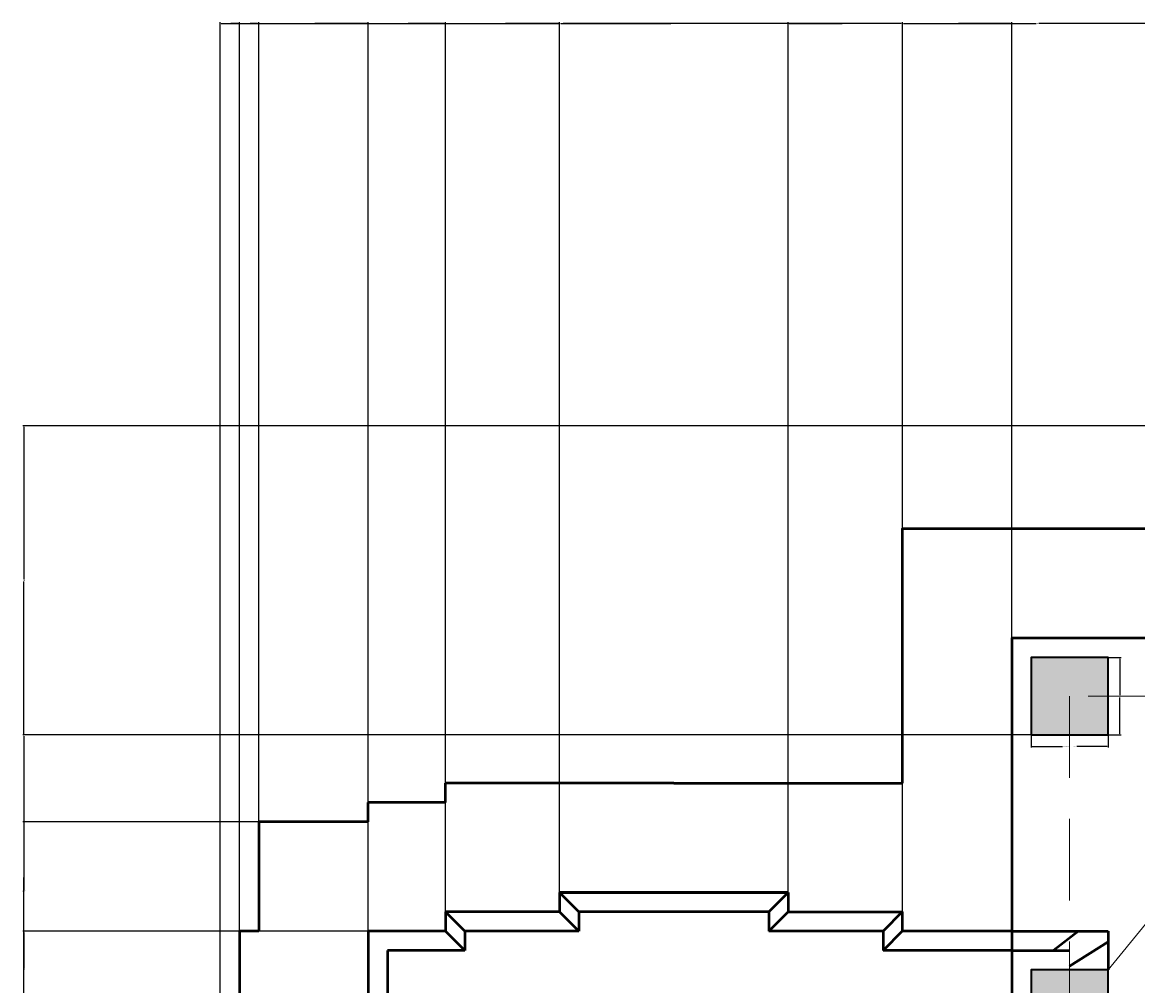
# Model space of a CAD drawing. Units: inches. Extents: x 386 to 107067, y -7 to 96314.
# Tile 5 of 10: x 592 to 766, y 1121 to 1271. Entities that reach past the tile are written whole.
import ezdxf

# ---------------------------------------------------------------- set-up
doc = ezdxf.new("R2010")
doc.units = ezdxf.units.IN
doc.linetypes.add('DASHED', pattern=[19.05, 12.7, -6.35])
for name, color, linetype, lineweight in [('A-ANNO-DIMS', 2, 'Continuous', 18), ('A-COLS', 1, 'Continuous', 35), ('A-FLOR-OVHD', 8, 'DASHED', 18), ('A-WALL', 7, 'Continuous', 50)]:
    doc.layers.add(name, color=color, linetype=linetype, lineweight=lineweight)
doc.styles.get("Standard").update_dxf_attribs({"font": 'arial.ttf'})
doc.dimstyles.get("Standard").update_dxf_attribs({"dimtxt": 0.18, "dimasz": 0.18, "dimexe": 0.18, "dimexo": 0.0625, "dimgap": 0.09, "dimtad": 0, "dimtih": 1, "dimtoh": 1, "dimdec": 4, "dimzin": 0, "dimdsep": 46, "dimtxsty": 'Standard', "dimcen": 0.09, "dimadec": 0, "dimazin": 0, "dimtfac": 1, "dimtdec": 4, "dimtofl": 0, "dimtmove": 0, "dimatfit": 3, "dimfxl": 1, "dimtolj": 1, "dimtzin": 0, "dimarcsym": 0})

# ---------------------------------------------------------------- blocks, each defined once
blk = doc.blocks.new('COL-300')
h = blk.add_hatch(color=256)
h.dxf.hatch_style = 1
h.paths.add_polyline_path([(761.03, 1172.09), (749.03, 1172.09), (749.03, 1160.09), (761.03, 1160.09)])
blk.add_lwpolyline([(749.03, 1160.09), (761.03, 1160.09), (761.03, 1172.09), (749.03, 1172.09)], close=True)
blk = doc.blocks.new('*D4')
at = {"layer": 'A-ANNO-DIMS', "color": 0, "lineweight": -2, "transparency": 16777216}
for p, q in [((749.03, 1160.03), (749.03, 1158.11)), ((761.03, 1160.03), (761.03, 1158.11)), ((749.21, 1158.29), (753.92, 1158.29)), ((760.85, 1158.29), (756.13, 1158.29))]:
    blk.add_line(p, q, dxfattribs=at)
at = {"layer": 'A-ANNO-DIMS', "color": 0, "transparency": 16777216}
for points in [[(749.21, 1158.32), (749.21, 1158.26), (749.03, 1158.29)], [(760.85, 1158.32), (760.85, 1158.26), (761.03, 1158.29)]]:
    blk.add_solid(points, dxfattribs=at)
at = {"layer": 'Defpoints', "color": 0, "transparency": 16777216}
for p in [(749.03, 1160.09), (761.03, 1160.09), (761.03, 1158.29)]:
    blk.add_point(p, dxfattribs=at)
at = {"layer": 'A-ANNO-DIMS', "color": 0, "transparency": 16777216, "insert": (755.03, 1158.29), "char_height": 0.18, "attachment_point": 5}
blk.add_mtext('\\A1;COLUMN 12 TYP.', dxfattribs=at)
blk = doc.blocks.new('*D5')
at = {"layer": 'A-ANNO-DIMS', "color": 0, "lineweight": -2, "transparency": 16777216}
for p, q in [((761.09, 1172.09), (763.01, 1172.09)), ((762.83, 1171.91), (762.83, 1166.27)), ((762.83, 1160.27), (762.83, 1165.91)), ((761.09, 1160.09), (763.01, 1160.09))]:
    blk.add_line(p, q, dxfattribs=at)
at = {"layer": 'A-ANNO-DIMS', "color": 0, "transparency": 16777216}
for points in [[(762.8, 1171.91), (762.86, 1171.91), (762.83, 1172.09)], [(762.8, 1160.27), (762.86, 1160.27), (762.83, 1160.09)]]:
    blk.add_solid(points, dxfattribs=at)
at = {"layer": 'Defpoints', "color": 0, "transparency": 16777216}
for p in [(761.03, 1172.09), (762.83, 1172.09), (761.03, 1160.09)]:
    blk.add_point(p, dxfattribs=at)
at = {"layer": 'A-ANNO-DIMS', "color": 0, "transparency": 16777216, "insert": (762.83, 1166.09), "char_height": 0.18, "attachment_point": 5}
blk.add_mtext('\\A1;12 TYP.', dxfattribs=at)
blk = doc.blocks.new('*D9')
at = {"layer": 'A-ANNO-DIMS', "color": 0, "lineweight": -2, "transparency": 16777216}
for p, q in [((623.03, 1117.65), (623.03, 1270.77)), ((623.21, 1270.59), (675.74, 1270.59)), ((728.85, 1270.59), (676.31, 1270.59)), ((729.03, 1152.65), (729.03, 1270.77))]:
    blk.add_line(p, q, dxfattribs=at)
at = {"layer": 'A-ANNO-DIMS', "color": 0, "transparency": 16777216}
for points in [[(623.21, 1270.62), (623.21, 1270.56), (623.03, 1270.59)], [(728.85, 1270.62), (728.85, 1270.56), (729.03, 1270.59)]]:
    blk.add_solid(points, dxfattribs=at)
at = {"layer": 'Defpoints', "color": 0, "transparency": 16777216}
for p in [(729.03, 1270.59), (729.03, 1152.59), (623.03, 1117.59)]:
    blk.add_point(p, dxfattribs=at)
at = {"layer": 'A-ANNO-DIMS', "color": 0, "transparency": 16777216, "insert": (676.03, 1270.59), "char_height": 0.18, "attachment_point": 5}
blk.add_mtext('\\A1;106', dxfattribs=at)
blk = doc.blocks.new('*D10')
at = {"layer": 'A-ANNO-DIMS', "color": 0, "lineweight": -2, "transparency": 16777216}
for p, q in [((729.03, 1192.15), (729.03, 1270.77)), ((729.21, 1270.59), (749.8, 1270.59)), ((770.85, 1270.59), (750.25, 1270.59)), ((771.03, 1240.15), (771.03, 1270.77))]:
    blk.add_line(p, q, dxfattribs=at)
at = {"layer": 'A-ANNO-DIMS', "color": 0, "transparency": 16777216}
for points in [[(729.21, 1270.62), (729.21, 1270.56), (729.03, 1270.59)], [(770.85, 1270.62), (770.85, 1270.56), (771.03, 1270.59)]]:
    blk.add_solid(points, dxfattribs=at)
at = {"layer": 'Defpoints', "color": 0, "transparency": 16777216}
for p in [(771.03, 1270.59), (771.03, 1240.09), (729.03, 1192.09)]:
    blk.add_point(p, dxfattribs=at)
at = {"layer": 'A-ANNO-DIMS', "color": 0, "transparency": 16777216, "insert": (750.03, 1270.59), "char_height": 0.18, "attachment_point": 5}
blk.add_mtext('\\A1;42', dxfattribs=at)
blk = doc.blocks.new('*D34')
at = {"layer": 'A-ANNO-DIMS', "color": 0, "lineweight": -2, "transparency": 16777216}
for p, q in [((748.96, 1160.09), (592.35, 1160.09)), ((592.53, 1159.91), (592.53, 1136.02)), ((592.53, 1111.77), (592.53, 1135.66)), ((748.96, 1111.59), (592.35, 1111.59))]:
    blk.add_line(p, q, dxfattribs=at)
at = {"layer": 'A-ANNO-DIMS', "color": 0, "transparency": 16777216}
for points in [[(592.5, 1159.91), (592.56, 1159.91), (592.53, 1160.09)], [(592.5, 1111.77), (592.56, 1111.77), (592.53, 1111.59)]]:
    blk.add_solid(points, dxfattribs=at)
at = {"layer": 'Defpoints', "color": 0, "transparency": 16777216}
for p in [(592.53, 1160.09), (749.03, 1160.09), (749.03, 1111.59)]:
    blk.add_point(p, dxfattribs=at)
at = {"layer": 'A-ANNO-DIMS', "color": 0, "transparency": 16777216, "insert": (592.53, 1135.84), "char_height": 0.18, "attachment_point": 5}
blk.add_mtext('\\A1;48.5', dxfattribs=at)
blk = doc.blocks.new('*D35')
at = {"layer": 'A-ANNO-DIMS', "color": 0, "lineweight": -2, "transparency": 16777216}
for p, q in [((790.96, 1208.09), (592.35, 1208.09)), ((592.53, 1207.91), (592.53, 1184.27)), ((592.53, 1160.27), (592.53, 1183.91)), ((748.96, 1160.09), (592.35, 1160.09))]:
    blk.add_line(p, q, dxfattribs=at)
at = {"layer": 'A-ANNO-DIMS', "color": 0, "transparency": 16777216}
for points in [[(592.5, 1207.91), (592.56, 1207.91), (592.53, 1208.09)], [(592.5, 1160.27), (592.56, 1160.27), (592.53, 1160.09)]]:
    blk.add_solid(points, dxfattribs=at)
at = {"layer": 'Defpoints', "color": 0, "transparency": 16777216}
for p in [(592.53, 1208.09), (791.03, 1208.09), (749.03, 1160.09)]:
    blk.add_point(p, dxfattribs=at)
at = {"layer": 'A-ANNO-DIMS', "color": 0, "transparency": 16777216, "insert": (592.53, 1184.09), "char_height": 0.18, "attachment_point": 5}
blk.add_mtext('\\A1;48', dxfattribs=at)
blk = doc.blocks.new('*D36')
at = {"layer": 'A-ANNO-DIMS', "color": 0, "lineweight": -2, "transparency": 16777216}
for p, q in [((623.03, 1117.65), (623.03, 1270.77)), ((623.21, 1270.59), (624.38, 1270.59)), ((625.85, 1270.59), (624.67, 1270.59)), ((626.03, 1129.65), (626.03, 1270.77))]:
    blk.add_line(p, q, dxfattribs=at)
at = {"layer": 'A-ANNO-DIMS', "color": 0, "transparency": 16777216}
for points in [[(623.21, 1270.62), (623.21, 1270.56), (623.03, 1270.59)], [(625.85, 1270.62), (625.85, 1270.56), (626.03, 1270.59)]]:
    blk.add_solid(points, dxfattribs=at)
at = {"layer": 'Defpoints', "color": 0, "transparency": 16777216}
for p in [(626.03, 1270.59), (626.03, 1129.59), (623.03, 1117.59)]:
    blk.add_point(p, dxfattribs=at)
at = {"layer": 'A-ANNO-DIMS', "color": 0, "transparency": 16777216, "insert": (624.53, 1270.59), "char_height": 0.18, "attachment_point": 5}
blk.add_mtext('\\A1;3', dxfattribs=at)
blk = doc.blocks.new('*D37')
at = {"layer": 'A-ANNO-DIMS', "color": 0, "lineweight": -2, "transparency": 16777216}
for p, q in [((626.03, 1129.65), (626.03, 1270.77)), ((626.21, 1270.59), (627.38, 1270.59)), ((628.85, 1270.59), (627.67, 1270.59)), ((629.03, 1146.65), (629.03, 1270.77))]:
    blk.add_line(p, q, dxfattribs=at)
at = {"layer": 'A-ANNO-DIMS', "color": 0, "transparency": 16777216}
for points in [[(626.21, 1270.62), (626.21, 1270.56), (626.03, 1270.59)], [(628.85, 1270.62), (628.85, 1270.56), (629.03, 1270.59)]]:
    blk.add_solid(points, dxfattribs=at)
at = {"layer": 'Defpoints', "color": 0, "transparency": 16777216}
for p in [(629.03, 1270.59), (629.03, 1146.59), (626.03, 1129.59)]:
    blk.add_point(p, dxfattribs=at)
at = {"layer": 'A-ANNO-DIMS', "color": 0, "transparency": 16777216, "insert": (627.53, 1270.59), "char_height": 0.18, "attachment_point": 5}
blk.add_mtext('\\A1;3', dxfattribs=at)
blk = doc.blocks.new('*D38')
at = {"layer": 'A-ANNO-DIMS', "color": 0, "lineweight": -2, "transparency": 16777216}
for p, q in [((629.03, 1146.65), (629.03, 1270.77)), ((629.21, 1270.59), (637.31, 1270.59)), ((645.85, 1270.59), (637.74, 1270.59)), ((646.03, 1149.65), (646.03, 1270.77))]:
    blk.add_line(p, q, dxfattribs=at)
at = {"layer": 'A-ANNO-DIMS', "color": 0, "transparency": 16777216}
for points in [[(629.21, 1270.62), (629.21, 1270.56), (629.03, 1270.59)], [(645.85, 1270.62), (645.85, 1270.56), (646.03, 1270.59)]]:
    blk.add_solid(points, dxfattribs=at)
at = {"layer": 'Defpoints', "color": 0, "transparency": 16777216}
for p in [(646.03, 1270.59), (646.03, 1149.59), (629.03, 1146.59)]:
    blk.add_point(p, dxfattribs=at)
at = {"layer": 'A-ANNO-DIMS', "color": 0, "transparency": 16777216, "insert": (637.53, 1270.59), "char_height": 0.18, "attachment_point": 5}
blk.add_mtext('\\A1;17', dxfattribs=at)
blk = doc.blocks.new('*D39')
at = {"layer": 'A-ANNO-DIMS', "color": 0, "lineweight": -2, "transparency": 16777216}
for p, q in [((646.03, 1129.65), (646.03, 1270.77)), ((646.21, 1270.59), (651.82, 1270.59)), ((657.85, 1270.59), (652.23, 1270.59)), ((658.03, 1132.65), (658.03, 1270.77))]:
    blk.add_line(p, q, dxfattribs=at)
at = {"layer": 'A-ANNO-DIMS', "color": 0, "transparency": 16777216}
for points in [[(646.21, 1270.62), (646.21, 1270.56), (646.03, 1270.59)], [(657.85, 1270.62), (657.85, 1270.56), (658.03, 1270.59)]]:
    blk.add_solid(points, dxfattribs=at)
at = {"layer": 'Defpoints', "color": 0, "transparency": 16777216}
for p in [(658.03, 1270.59), (658.03, 1132.59), (646.03, 1129.59)]:
    blk.add_point(p, dxfattribs=at)
at = {"layer": 'A-ANNO-DIMS', "color": 0, "transparency": 16777216, "insert": (652.03, 1270.59), "char_height": 0.18, "attachment_point": 5}
blk.add_mtext('\\A1;12', dxfattribs=at)
blk = doc.blocks.new('*D40')
at = {"layer": 'A-ANNO-DIMS', "color": 0, "lineweight": -2, "transparency": 16777216}
for p, q in [((658.03, 1132.65), (658.03, 1270.77)), ((658.21, 1270.59), (666.44, 1270.59)), ((675.59, 1270.59), (667.35, 1270.59)), ((675.77, 1135.65), (675.77, 1270.77))]:
    blk.add_line(p, q, dxfattribs=at)
at = {"layer": 'A-ANNO-DIMS', "color": 0, "transparency": 16777216}
for points in [[(658.21, 1270.62), (658.21, 1270.56), (658.03, 1270.59)], [(675.59, 1270.62), (675.59, 1270.56), (675.77, 1270.59)]]:
    blk.add_solid(points, dxfattribs=at)
at = {"layer": 'Defpoints', "color": 0, "transparency": 16777216}
for p in [(675.77, 1270.59), (675.77, 1135.59), (658.03, 1132.59)]:
    blk.add_point(p, dxfattribs=at)
at = {"layer": 'A-ANNO-DIMS', "color": 0, "transparency": 16777216, "insert": (666.9, 1270.59), "char_height": 0.18, "attachment_point": 5}
blk.add_mtext('\\A1;17.748', dxfattribs=at)
blk = doc.blocks.new('*D41')
at = {"layer": 'A-ANNO-DIMS', "color": 0, "lineweight": -2, "transparency": 16777216}
for p, q in [((675.77, 1135.65), (675.77, 1270.77)), ((675.95, 1270.59), (693.06, 1270.59)), ((711.09, 1270.59), (693.98, 1270.59)), ((711.27, 1135.65), (711.27, 1270.77))]:
    blk.add_line(p, q, dxfattribs=at)
at = {"layer": 'A-ANNO-DIMS', "color": 0, "transparency": 16777216}
for points in [[(675.95, 1270.62), (675.95, 1270.56), (675.77, 1270.59)], [(711.09, 1270.62), (711.09, 1270.56), (711.27, 1270.59)]]:
    blk.add_solid(points, dxfattribs=at)
at = {"layer": 'Defpoints', "color": 0, "transparency": 16777216}
for p in [(711.27, 1270.59), (675.77, 1135.59), (711.27, 1135.59)]:
    blk.add_point(p, dxfattribs=at)
at = {"layer": 'A-ANNO-DIMS', "color": 0, "transparency": 16777216, "insert": (693.52, 1270.59), "char_height": 0.18, "attachment_point": 5}
blk.add_mtext('\\A1;35.496', dxfattribs=at)
blk = doc.blocks.new('*D42')
at = {"layer": 'A-ANNO-DIMS', "color": 0, "lineweight": -2, "transparency": 16777216}
for p, q in [((711.27, 1135.65), (711.27, 1270.77)), ((711.45, 1270.59), (719.69, 1270.59)), ((728.85, 1270.59), (720.6, 1270.59)), ((729.03, 1132.65), (729.03, 1270.77))]:
    blk.add_line(p, q, dxfattribs=at)
at = {"layer": 'A-ANNO-DIMS', "color": 0, "transparency": 16777216}
for points in [[(711.45, 1270.62), (711.45, 1270.56), (711.27, 1270.59)], [(728.85, 1270.62), (728.85, 1270.56), (729.03, 1270.59)]]:
    blk.add_solid(points, dxfattribs=at)
at = {"layer": 'Defpoints', "color": 0, "transparency": 16777216}
for p in [(729.03, 1270.59), (711.27, 1135.59), (729.03, 1132.59)]:
    blk.add_point(p, dxfattribs=at)
at = {"layer": 'A-ANNO-DIMS', "color": 0, "transparency": 16777216, "insert": (720.15, 1270.59), "char_height": 0.18, "attachment_point": 5}
blk.add_mtext('\\A1;17.756', dxfattribs=at)
blk = doc.blocks.new('*D43')
at = {"layer": 'A-ANNO-DIMS', "color": 0, "lineweight": -2, "transparency": 16777216}
for p, q in [((729.03, 1129.65), (729.03, 1270.77)), ((729.21, 1270.59), (737.31, 1270.59)), ((745.85, 1270.59), (737.74, 1270.59)), ((746.03, 1129.65), (746.03, 1270.77))]:
    blk.add_line(p, q, dxfattribs=at)
at = {"layer": 'A-ANNO-DIMS', "color": 0, "transparency": 16777216}
for points in [[(729.21, 1270.62), (729.21, 1270.56), (729.03, 1270.59)], [(745.85, 1270.62), (745.85, 1270.56), (746.03, 1270.59)]]:
    blk.add_solid(points, dxfattribs=at)
at = {"layer": 'Defpoints', "color": 0, "transparency": 16777216}
for p in [(746.03, 1270.59), (729.03, 1129.59), (746.03, 1129.59)]:
    blk.add_point(p, dxfattribs=at)
at = {"layer": 'A-ANNO-DIMS', "color": 0, "transparency": 16777216, "insert": (737.53, 1270.59), "char_height": 0.18, "attachment_point": 5}
blk.add_mtext('\\A1;17', dxfattribs=at)
blk = doc.blocks.new('*D47')
at = {"layer": 'A-ANNO-DIMS', "color": 0, "lineweight": -2, "transparency": 16777216}
for p, q in [((625.96, 1129.59), (592.35, 1129.59)), ((592.53, 1129.41), (592.53, 1123.77)), ((592.53, 1117.77), (592.53, 1123.41)), ((625.96, 1117.59), (592.35, 1117.59))]:
    blk.add_line(p, q, dxfattribs=at)
at = {"layer": 'A-ANNO-DIMS', "color": 0, "transparency": 16777216}
for points in [[(592.5, 1129.41), (592.56, 1129.41), (592.53, 1129.59)], [(592.5, 1117.77), (592.56, 1117.77), (592.53, 1117.59)]]:
    blk.add_solid(points, dxfattribs=at)
at = {"layer": 'Defpoints', "color": 0, "transparency": 16777216}
for p in [(592.53, 1129.59), (626.03, 1129.59), (626.03, 1117.59)]:
    blk.add_point(p, dxfattribs=at)
at = {"layer": 'A-ANNO-DIMS', "color": 0, "transparency": 16777216, "insert": (592.53, 1123.59), "char_height": 0.18, "attachment_point": 5}
blk.add_mtext('\\A1;12', dxfattribs=at)
blk = doc.blocks.new('*D48')
at = {"layer": 'A-ANNO-DIMS', "color": 0, "lineweight": -2, "transparency": 16777216}
for p, q in [((628.96, 1146.59), (592.35, 1146.59)), ((592.53, 1146.41), (592.53, 1138.27)), ((592.53, 1129.77), (592.53, 1137.91)), ((628.96, 1129.59), (592.35, 1129.59))]:
    blk.add_line(p, q, dxfattribs=at)
at = {"layer": 'A-ANNO-DIMS', "color": 0, "transparency": 16777216}
for points in [[(592.5, 1146.41), (592.56, 1146.41), (592.53, 1146.59)], [(592.5, 1129.77), (592.56, 1129.77), (592.53, 1129.59)]]:
    blk.add_solid(points, dxfattribs=at)
at = {"layer": 'Defpoints', "color": 0, "transparency": 16777216}
for p in [(592.53, 1146.59), (629.03, 1146.59), (629.03, 1129.59)]:
    blk.add_point(p, dxfattribs=at)
at = {"layer": 'A-ANNO-DIMS', "color": 0, "transparency": 16777216, "insert": (592.53, 1138.09), "char_height": 0.18, "attachment_point": 5}
blk.add_mtext('\\A1;17', dxfattribs=at)
blk = doc.blocks.new('*D51')
at = {"layer": 'A-ANNO-DIMS', "color": 0, "lineweight": -2, "transparency": 16777216}
for p, q in [((645.96, 1129.59), (592.35, 1129.59)), ((592.53, 1129.41), (592.53, 1123.77)), ((592.53, 1117.77), (592.53, 1123.41)), ((645.96, 1117.59), (592.35, 1117.59))]:
    blk.add_line(p, q, dxfattribs=at)
at = {"layer": 'A-ANNO-DIMS', "color": 0, "transparency": 16777216}
for points in [[(592.5, 1129.41), (592.56, 1129.41), (592.53, 1129.59)], [(592.5, 1117.77), (592.56, 1117.77), (592.53, 1117.59)]]:
    blk.add_solid(points, dxfattribs=at)
at = {"layer": 'Defpoints', "color": 0, "transparency": 16777216}
for p in [(592.53, 1129.59), (646.03, 1129.59), (646.03, 1117.59)]:
    blk.add_point(p, dxfattribs=at)
at = {"layer": 'A-ANNO-DIMS', "color": 0, "transparency": 16777216, "insert": (592.53, 1123.59), "char_height": 0.18, "attachment_point": 5}
blk.add_mtext('\\A1;12', dxfattribs=at)

msp = doc.modelspace()

# ---------------------------------------------------------------- linework, layer by layer
at = {"layer": 'A-FLOR-OVHD'}
msp.add_line((791.0252, 1160.0919), (761.0252, 1123.5919), dxfattribs=at)
msp.add_lwpolyline([(755.0252, 998.0919), (923.0252, 998.0919), (923.0252, 1166.0919), (755.0252, 1166.0919)], close=True, dxfattribs=at)
at = {"layer": 'A-WALL'}
for p, q in [((658.0252, 1149.5919), (658.0252, 1152.5919)), ((693.5212, 1152.5919), (729.0252, 1152.5919)), ((646.0252, 1146.5919), (646.0252, 1149.5919)), ((711.2692, 1135.5919), (675.7732, 1135.5919)), ((675.7732, 1135.5919), (675.7732, 1132.5919)), ((675.7732, 1135.5919), (693.5212, 1135.5919)), ((675.7732, 1135.5919), (678.7732, 1132.5919)), ((693.5212, 1135.5919), (711.2692, 1135.5919)), ((711.2692, 1135.5919), (708.2692, 1132.5919)), ((711.2692, 1135.5919), (711.2692, 1132.5919)), ((675.7732, 1132.5919), (658.0252, 1132.5919)), ((658.0252, 1132.5919), (661.0252, 1129.5919)), ((675.7732, 1132.5919), (678.7732, 1129.5919)), ((678.7732, 1132.5919), (678.7732, 1129.5919)), ((708.2692, 1132.5919), (678.7732, 1132.5919)), ((708.2692, 1132.5919), (708.2692, 1129.5919)), ((711.2692, 1132.5919), (708.2692, 1129.5919)), ((729.0252, 1132.5919), (726.0252, 1129.5919)), ((629.0252, 1129.5919), (626.0252, 1129.5919)), ((658.0252, 1129.5919), (646.0252, 1129.5919)), ((658.0252, 1129.5919), (661.0252, 1126.5919)), ((678.7732, 1129.5919), (661.0252, 1129.5919)), ((726.0252, 1129.5919), (708.2692, 1129.5919)), ((729.0252, 1129.5919), (726.0252, 1126.5919)), ((746.0252, 1129.5919), (729.0252, 1129.5919)), ((746.0252, 1129.5919), (761.0252, 1129.5919)), ((756.4228, 1129.5919), (752.5267, 1126.5919)), ((761.0252, 1129.5919), (761.0252, 1123.5919)), ((661.0252, 1126.5919), (649.0252, 1126.5919)), ((746.0252, 1126.5919), (726.0252, 1126.5919)), ((746.0252, 1126.5919), (755.0252, 1126.5919)), ((761.0252, 1127.9205), (755.0252, 1124.1428))]:
    msp.add_line(p, q, dxfattribs=at)
for points in [[(771.0252, 1192.0919), (729.0252, 1192.0919), (729.0252, 1152.5919)], [(788.0252, 1175.0919), (746.0252, 1175.0919), (746.0252, 989.0919), (788.0252, 989.0919)], [(693.5212, 1152.5919), (658.0252, 1152.5919)], [(658.0252, 1149.5919), (646.0252, 1149.5919)], [(646.0252, 1146.5919), (629.0252, 1146.5919), (629.0252, 1129.5919)], [(658.0252, 1132.5919), (658.0252, 1129.5919)], [(711.2692, 1132.5919), (729.0252, 1132.5919), (729.0252, 1129.5919)], [(626.0252, 1129.5919), (626.0252, 1117.5919)], [(646.0252, 1129.5919), (646.0252, 1117.5919)], [(661.0252, 1129.5919), (661.0252, 1126.5919)], [(726.0252, 1129.5919), (726.0252, 1126.5919)], [(649.0252, 1126.5919), (649.0252, 1114.5919)]]:
    msp.add_lwpolyline(points, dxfattribs=at)

# ---------------------------------------------------------------- block references
at = {"layer": 'A-COLS'}
for p in [(0, 0), (0, -48.5)]:
    msp.add_blockref('COL-300', p, dxfattribs=at)

# ---------------------------------------------------------------- dimensions: what is measured, and where the dimension line sits
at = {"layer": 'A-ANNO-DIMS'}
for base, p1, p2, override, picture, middle in [((729.0252, 1270.5919), (623.0252, 1117.5919), (729.0252, 1152.5919), {"dimdec": 0, "dimlfac": 1, "dimrnd": 0, "dimzin": 0, "dimdsep": 46, "dimlunit": 2}, '*D9', (676.0252, 1270.5919)), ((626.0252, 1270.5919), (623.0252, 1117.5919), (626.0252, 1129.5919), {"dimdec": 0, "dimlfac": 1, "dimrnd": 0, "dimzin": 0, "dimdsep": 46, "dimlunit": 2}, '*D36', (624.5252, 1270.5919)), ((629.0252, 1270.5919), (626.0252, 1129.5919), (629.0252, 1146.5919), {"dimdec": 0, "dimlfac": 1, "dimrnd": 0, "dimzin": 0, "dimdsep": 46, "dimlunit": 2}, '*D37', (627.5252, 1270.5919)), ((646.0252, 1270.5919), (629.0252, 1146.5919), (646.0252, 1149.5919), {"dimdec": 0, "dimlfac": 1, "dimrnd": 0, "dimzin": 0, "dimdsep": 46, "dimlunit": 2}, '*D38', (637.5252, 1270.5919)), ((658.0252, 1270.5919), (646.0252, 1129.5919), (658.0252, 1132.5919), {"dimdec": 0, "dimlfac": 1, "dimrnd": 0, "dimzin": 0, "dimdsep": 46, "dimlunit": 2}, '*D39', (652.0252, 1270.5919)), ((675.7732, 1270.5919), (658.0252, 1132.5919), (675.7732, 1135.5919), {"dimdec": 3, "dimlfac": 1, "dimrnd": 0, "dimzin": 0, "dimdsep": 46, "dimlunit": 2}, '*D40', (666.8992, 1270.5919)), ((711.2692, 1270.5919), (675.7732, 1135.5919), (711.2692, 1135.5919), {"dimdec": 3, "dimlfac": 1, "dimrnd": 0, "dimzin": 0, "dimdsep": 46, "dimlunit": 2}, '*D41', (693.5212, 1270.5919)), ((729.0252, 1270.5919), (711.2692, 1135.5919), (729.0252, 1132.5919), {"dimdec": 3, "dimlfac": 1, "dimrnd": 0, "dimzin": 0, "dimdsep": 46, "dimlunit": 2}, '*D42', (720.1472, 1270.5919)), ((771.0252, 1270.5919), (729.0252, 1192.0919), (771.0252, 1240.0919), {"dimdec": 0, "dimlfac": 1, "dimrnd": 0, "dimzin": 0, "dimdsep": 46, "dimlunit": 2}, '*D10', (750.0252, 1270.5919)), ((746.0252, 1270.5919), (729.0252, 1129.5919), (746.0252, 1129.5919), {"dimdec": 0, "dimlfac": 1, "dimrnd": 0, "dimzin": 0, "dimdsep": 46, "dimlunit": 2}, '*D43', (737.5252, 1270.5919))]:
    dim = msp.add_linear_dim(base=base, p1=p1, p2=p2, dimstyle='Standard', override=override, dxfattribs=at)
    dim.commit()
    dim.dimension.update_dxf_attribs({"geometry": picture, "text_midpoint": middle})
for base, p1, p2, override, picture, middle in [((592.5252, 1208.0919), (749.0252, 1160.0919), (791.0252, 1208.0919), {"dimdec": 0, "dimlfac": 1, "dimrnd": 0, "dimzin": 0, "dimdsep": 46, "dimlunit": 2}, '*D35', (592.5252, 1184.0919)), ((592.5252, 1160.0919), (749.0252, 1111.5919), (749.0252, 1160.0919), {"dimdec": 1, "dimlfac": 1, "dimrnd": 0, "dimzin": 0, "dimdsep": 46, "dimlunit": 2}, '*D34', (592.5252, 1135.8419)), ((592.5252, 1146.5919), (629.0252, 1129.5919), (629.0252, 1146.5919), {"dimdec": 0, "dimlfac": 1, "dimrnd": 0, "dimzin": 0, "dimdsep": 46, "dimlunit": 2}, '*D48', (592.5252, 1138.0919)), ((592.5252, 1129.5919), (626.0252, 1117.5919), (626.0252, 1129.5919), {"dimdec": 0, "dimlfac": 1, "dimrnd": 0, "dimzin": 0, "dimdsep": 46, "dimlunit": 2}, '*D47', (592.5252, 1123.5919)), ((592.5252, 1129.5919), (646.0252, 1117.5919), (646.0252, 1129.5919), {"dimdec": 0, "dimlfac": 1, "dimrnd": 0, "dimzin": 0, "dimdsep": 46, "dimlunit": 2}, '*D51', (592.5252, 1123.5919))]:
    dim = msp.add_linear_dim(base=base, p1=p1, p2=p2, angle=90, dimstyle='Standard', override=override, dxfattribs=at)
    dim.commit()
    dim.dimension.update_dxf_attribs({"geometry": picture, "text_midpoint": middle})
dim = msp.add_linear_dim(base=(762.8252, 1172.0919), p1=(761.0252, 1160.0919), p2=(761.0252, 1172.0919), angle=90, text='<> TYP.', dimstyle='Standard', override={"dimdec": 0, "dimlfac": 1, "dimrnd": 0, "dimzin": 0, "dimdsep": 46, "dimlunit": 2}, dxfattribs=at)
dim.commit()
dim.dimension.update_dxf_attribs({"geometry": '*D5', "text_midpoint": (762.8252, 1166.0919)})
dim = msp.add_linear_dim(base=(761.0252, 1158.2919), p1=(749.0252, 1160.0919), p2=(761.0252, 1160.0919), text='COLUMN <> TYP.', dimstyle='Standard', override={"dimdec": 0, "dimlfac": 1, "dimrnd": 0, "dimzin": 0, "dimdsep": 46, "dimlunit": 2}, dxfattribs=at)
dim.commit()
dim.dimension.update_dxf_attribs({"geometry": '*D4', "text_midpoint": (755.0252, 1158.2919)})

doc.saveas('drawing.dxf')
